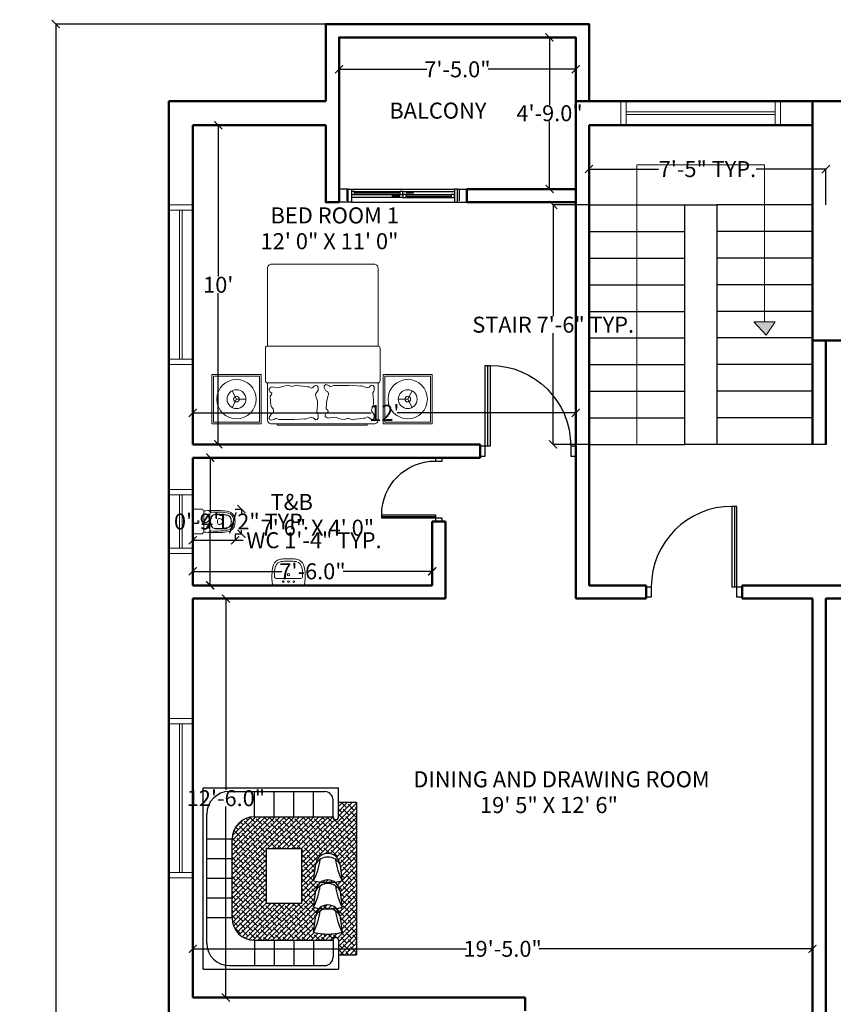
# Model space of a CAD drawing. Units: inches. Extents: x 147 to 1638, y 107 to 941.
# Tile 16 of 17: x 1062 to 1368, y 570 to 940. Entities that reach past the tile are written whole.
import ezdxf

# ---------------------------------------------------------------- set-up
doc = ezdxf.new("R2010")
doc.units = ezdxf.units.IN
doc.header["$MEASUREMENT"] = 0
for name, color, linetype, lineweight in [('A-ANNO-DIMS', 2, 'Continuous', 15), ('A-ANNO-SYMB', 7, 'Continuous', 18), ('A-AREA-IDEN', 7, 'Continuous', 18), ('A-Door', 150, 'Continuous', 25), ('A-FLOR-FIXT', 9, 'Continuous', 18), ('A-FLOR-STRS', 7, 'Continuous', 25), ('furniture', 50, 'Continuous', 18), ('HAT', 9, 'Continuous', 0), ('walls', 7, 'Continuous', 50), ('windows', 3, 'Continuous', 20)]:
    doc.layers.add(name, color=color, linetype=linetype, lineweight=lineweight)
for name, color, linetype in [('A-Glaz', 92, 'Continuous'), ('FUR', 42, 'Continuous'), ('NT', 1, 'Continuous'), ('Win', 152, 'Continuous')]:
    doc.layers.add(name, color=color, linetype=linetype)
doc.styles.get("Standard").update_dxf_attribs({"font": 'arial.ttf'})
doc.dimstyles.get("Standard").update_dxf_attribs({"dimtxt": 6, "dimasz": 3, "dimexe": 0.18, "dimexo": 0.0625, "dimgap": 0.09, "dimtad": 0, "dimtih": 1, "dimtoh": 1, "dimdec": 1, "dimzin": 0, "dimdsep": 46, "dimlunit": 3, "dimtxsty": 'Standard', "dimblk": 'ARCHTICK', "dimcen": 0.09, "dimadec": 0, "dimazin": 0, "dimtfac": 1, "dimtdec": 1, "dimtofl": 0, "dimtmove": 0, "dimatfit": 3, "dimfxl": 1, "dimtolj": 1, "dimtzin": 0, "dimarcsym": 0})

# ---------------------------------------------------------------- blocks, each defined once
blk = doc.blocks.new('A$C087A3AA9')
at = {"layer": 'A-Door'}
for points in [[(852.6, 94.7), (852.6, 852.6), (805.3, 852.6), (805.3, 94.7)], [(47.4, 94.7), (47.4, 0), (0, 0), (0, 94.7)], [(900, 94.7), (900, 0), (852.6, 0), (852.6, 94.7)]]:
    blk.add_lwpolyline(points, close=True, dxfattribs=at)
at = {"layer": 'A-Glaz'}
blk.add_line((828.9, 852.6), (828.9, 94.7), dxfattribs=at)
at = {"layer": 'NT'}
blk.add_arc((805.3, 94.7), 757.9, 90, 180, dxfattribs=at)
blk = doc.blocks.new('_ArchTick')
at = {"color": 0, "linetype": 'ByBlock', "const_width": 0.15}
blk.add_lwpolyline([(-0.5, -0.5), (0.5, 0.5)], dxfattribs=at)
blk = doc.blocks.new('*D49')
at = {"layer": 'A-ANNO-DIMS', "color": 0, "lineweight": -2, "transparency": 16777216}
for p, q in [((1132.08, 900.72), (1136.52, 900.72)), ((1136.34, 900.72), (1136.34, 843.87)), ((1136.34, 780.72), (1136.34, 837.56)), ((1132.08, 780.72), (1136.52, 780.72))]:
    blk.add_line(p, q, dxfattribs=at)
at = {"layer": 'Defpoints', "color": 0, "lineweight": -2, "transparency": 16777216}
for p in [(1132.02, 900.72), (1132.02, 780.72), (1136.34, 780.72)]:
    blk.add_point(p, dxfattribs=at)
at = {"layer": 'A-ANNO-DIMS', "color": 0, "lineweight": -2, "transparency": 16777216, "xscale": 3, "yscale": 3, "zscale": 3}
for p, rotation in [((1136.34, 900.72), 90), ((1136.34, 780.72), 270)]:
    blk.add_blockref('_ArchTick', p, dxfattribs=dict(at, rotation=rotation))
at = {"layer": 'A-ANNO-DIMS', "color": 0, "transparency": 16777216, "insert": (1136.34, 840.72), "char_height": 6, "attachment_point": 5}
blk.add_mtext("\\A1;10'", dxfattribs=at)
blk = doc.blocks.new('*D50')
at = {"layer": 'A-ANNO-DIMS', "color": 0, "lineweight": -2, "transparency": 16777216}
for p, q in [((1126.77, 788.89), (1126.77, 792.75)), ((1126.77, 792.57), (1193.87, 792.57)), ((1270.77, 792.57), (1203.67, 792.57)), ((1270.77, 788.89), (1270.77, 792.75))]:
    blk.add_line(p, q, dxfattribs=at)
at = {"layer": 'Defpoints', "color": 0, "lineweight": -2, "transparency": 16777216}
for p in [(1270.77, 792.57), (1126.77, 788.82), (1270.77, 788.82)]:
    blk.add_point(p, dxfattribs=at)
at = {"layer": 'A-ANNO-DIMS', "color": 0, "lineweight": -2, "transparency": 16777216, "xscale": 3, "yscale": 3, "zscale": 3, "rotation": 180}
blk.add_blockref('_ArchTick', (1126.77, 792.57), dxfattribs=at)
at = {"layer": 'A-ANNO-DIMS', "color": 0, "lineweight": -2, "transparency": 16777216, "xscale": 3, "yscale": 3, "zscale": 3}
blk.add_blockref('_ArchTick', (1270.77, 792.57), dxfattribs=at)
at = {"layer": 'A-ANNO-DIMS', "color": 0, "transparency": 16777216, "insert": (1198.77, 792.57), "char_height": 6, "attachment_point": 5}
blk.add_mtext("\\A1;12'", dxfattribs=at)
blk = doc.blocks.new('*D51')
at = {"layer": 'A-ANNO-DIMS', "color": 0, "lineweight": -2, "transparency": 16777216}
for p, q in [((1266.32, 933.72), (1260.72, 933.72)), ((1260.9, 933.72), (1260.9, 908.37)), ((1260.9, 876.72), (1260.9, 902.06)), ((1266.32, 876.72), (1260.72, 876.72))]:
    blk.add_line(p, q, dxfattribs=at)
at = {"layer": 'Defpoints', "color": 0, "lineweight": -2, "transparency": 16777216}
for p in [(1266.38, 933.72), (1260.9, 876.72), (1266.38, 876.72)]:
    blk.add_point(p, dxfattribs=at)
at = {"layer": 'A-ANNO-DIMS', "color": 0, "lineweight": -2, "transparency": 16777216, "xscale": 3, "yscale": 3, "zscale": 3}
for p, rotation in [((1260.9, 933.72), 90), ((1260.9, 876.72), 270)]:
    blk.add_blockref('_ArchTick', p, dxfattribs=dict(at, rotation=rotation))
at = {"layer": 'A-ANNO-DIMS', "color": 0, "transparency": 16777216, "insert": (1260.9, 905.22), "char_height": 6, "attachment_point": 5}
blk.add_mtext('\\A1;4\'-9.0"', dxfattribs=at)
blk = doc.blocks.new('*D52')
at = {"layer": 'A-ANNO-DIMS', "color": 0, "lineweight": -2, "transparency": 16777216}
for p, q in [((1181.77, 928.29), (1181.77, 921.54)), ((1270.77, 928.29), (1270.77, 921.54)), ((1181.77, 921.72), (1214.73, 921.72)), ((1270.77, 921.72), (1237.8, 921.72))]:
    blk.add_line(p, q, dxfattribs=at)
at = {"layer": 'Defpoints', "color": 0, "lineweight": -2, "transparency": 16777216}
for p in [(1181.77, 928.35), (1270.77, 928.35), (1270.77, 921.72)]:
    blk.add_point(p, dxfattribs=at)
at = {"layer": 'A-ANNO-DIMS', "color": 0, "lineweight": -2, "transparency": 16777216, "xscale": 3, "yscale": 3, "zscale": 3, "rotation": 180}
blk.add_blockref('_ArchTick', (1181.77, 921.72), dxfattribs=at)
at = {"layer": 'A-ANNO-DIMS', "color": 0, "lineweight": -2, "transparency": 16777216, "xscale": 3, "yscale": 3, "zscale": 3}
blk.add_blockref('_ArchTick', (1270.77, 921.72), dxfattribs=at)
at = {"layer": 'A-ANNO-DIMS', "color": 0, "transparency": 16777216, "insert": (1226.27, 921.72), "char_height": 6, "attachment_point": 5}
blk.add_mtext('\\A1;7\'-5.0"', dxfattribs=at)
blk = doc.blocks.new('*D55')
at = {"layer": 'A-ANNO-DIMS', "color": 0, "lineweight": -2, "transparency": 16777216}
for p, q in [((1126.77, 733.06), (1126.77, 733.17)), ((1126.77, 732.99), (1160.23, 732.99)), ((1216.77, 732.99), (1183.3, 732.99)), ((1216.77, 733.06), (1216.77, 733.17))]:
    blk.add_line(p, q, dxfattribs=at)
at = {"layer": 'Defpoints', "color": 0, "lineweight": -2, "transparency": 16777216}
for p in [(1126.77, 732.99), (1216.77, 732.99), (1216.77, 732.99)]:
    blk.add_point(p, dxfattribs=at)
at = {"layer": 'A-ANNO-DIMS', "color": 0, "lineweight": -2, "transparency": 16777216, "xscale": 3, "yscale": 3, "zscale": 3, "rotation": 180}
blk.add_blockref('_ArchTick', (1126.77, 732.99), dxfattribs=at)
at = {"layer": 'A-ANNO-DIMS', "color": 0, "lineweight": -2, "transparency": 16777216, "xscale": 3, "yscale": 3, "zscale": 3}
blk.add_blockref('_ArchTick', (1216.77, 732.99), dxfattribs=at)
at = {"layer": 'A-ANNO-DIMS', "color": 0, "transparency": 16777216, "insert": (1171.77, 732.99), "char_height": 6, "attachment_point": 5}
blk.add_mtext('\\A1;7\'-6.0"', dxfattribs=at)
blk = doc.blocks.new('*D56')
at = {"layer": 'A-ANNO-DIMS', "color": 0, "lineweight": -2, "transparency": 16777216}
for p, q in [((1133.31, 775.72), (1133.31, 754.81)), ((1133.37, 775.72), (1133.49, 775.72)), ((1133.31, 727.72), (1133.31, 748.63)), ((1133.37, 727.72), (1133.49, 727.72))]:
    blk.add_line(p, q, dxfattribs=at)
at = {"layer": 'Defpoints', "color": 0, "lineweight": -2, "transparency": 16777216}
for p in [(1133.31, 775.72), (1133.31, 727.72), (1133.31, 727.72)]:
    blk.add_point(p, dxfattribs=at)
at = {"layer": 'A-ANNO-DIMS', "color": 0, "lineweight": -2, "transparency": 16777216, "xscale": 3, "yscale": 3, "zscale": 3}
for p, rotation in [((1133.31, 775.72), 90), ((1133.31, 727.72), 270)]:
    blk.add_blockref('_ArchTick', p, dxfattribs=dict(at, rotation=rotation))
at = {"layer": 'A-ANNO-DIMS', "color": 0, "transparency": 16777216, "insert": (1133.31, 751.72), "char_height": 6, "attachment_point": 5}
blk.add_mtext("\\A1;4'", dxfattribs=at)
blk = doc.blocks.new('*D57')
at = {"layer": 'A-ANNO-DIMS', "color": 0, "lineweight": -2, "transparency": 16777216}
for p, q in [((1140.05, 722.72), (1139.05, 722.72)), ((1139.23, 722.72), (1139.23, 650.87)), ((1139.23, 572.72), (1139.23, 644.56)), ((1140.05, 572.72), (1139.05, 572.72))]:
    blk.add_line(p, q, dxfattribs=at)
at = {"layer": 'Defpoints', "color": 0, "lineweight": -2, "transparency": 16777216}
for p in [(1140.11, 722.72), (1139.23, 572.72), (1140.11, 572.72)]:
    blk.add_point(p, dxfattribs=at)
at = {"layer": 'A-ANNO-DIMS', "color": 0, "lineweight": -2, "transparency": 16777216, "xscale": 3, "yscale": 3, "zscale": 3}
for p, rotation in [((1139.23, 722.72), 90), ((1139.23, 572.72), 270)]:
    blk.add_blockref('_ArchTick', p, dxfattribs=dict(at, rotation=rotation))
at = {"layer": 'A-ANNO-DIMS', "color": 0, "transparency": 16777216, "insert": (1139.23, 647.72), "char_height": 6, "attachment_point": 5}
blk.add_mtext('\\A1;12\'-6.0"', dxfattribs=at)
blk = doc.blocks.new('*D58')
at = {"layer": 'A-ANNO-DIMS', "color": 0, "lineweight": -2, "transparency": 16777216}
for p, q in [((1126.77, 585.3), (1126.77, 591.26)), ((1126.77, 591.08), (1229.66, 591.08)), ((1359.77, 591.08), (1256.88, 591.08)), ((1359.77, 585.3), (1359.77, 591.26))]:
    blk.add_line(p, q, dxfattribs=at)
at = {"layer": 'Defpoints', "color": 0, "lineweight": -2, "transparency": 16777216}
for p in [(1359.77, 591.08), (1126.77, 585.23), (1359.77, 585.23)]:
    blk.add_point(p, dxfattribs=at)
at = {"layer": 'A-ANNO-DIMS', "color": 0, "lineweight": -2, "transparency": 16777216, "xscale": 3, "yscale": 3, "zscale": 3, "rotation": 180}
blk.add_blockref('_ArchTick', (1126.77, 591.08), dxfattribs=at)
at = {"layer": 'A-ANNO-DIMS', "color": 0, "lineweight": -2, "transparency": 16777216, "xscale": 3, "yscale": 3, "zscale": 3}
blk.add_blockref('_ArchTick', (1359.77, 591.08), dxfattribs=at)
at = {"layer": 'A-ANNO-DIMS', "color": 0, "transparency": 16777216, "insert": (1243.27, 591.08), "char_height": 6, "attachment_point": 5}
blk.add_mtext('\\A1;19\'-5.0"', dxfattribs=at)
blk = doc.blocks.new('MAT-P14')
for p, q in [((-1.337, 1.348), (-1.337, 1.948)), ((-1.337, 1.948), (-0.737, 1.948)), ((-1.317, 1.928), (-0.757, 1.928)), ((-1.317, 1.368), (-1.317, 1.928)), ((-0.757, 1.368), (-0.757, 1.928)), ((-0.737, 1.348), (-0.737, 1.948)), ((0.625, 1.95), (-0.625, 1.95)), ((0.753, 1.348), (0.753, 1.948)), ((1.353, 1.948), (0.753, 1.948)), ((1.333, 1.928), (0.773, 1.928)), ((0.773, 1.368), (0.773, 1.928)), ((1.333, 1.368), (1.333, 1.928)), ((1.353, 1.348), (1.353, 1.948)), ((-1.037, 1.648), (-1.091, 1.749)), ((1.053, 1.648), (1.108, 1.749)), ((-1.037, 1.648), (-1.091, 1.547)), ((-1.037, 1.648), (-0.922, 1.648)), ((1.053, 1.648), (0.938, 1.648)), ((1.053, 1.648), (1.108, 1.547)), ((-1.337, 1.348), (-0.737, 1.348)), ((-1.317, 1.368), (-0.757, 1.368)), ((1.353, 1.348), (0.753, 1.348)), ((1.333, 1.368), (0.773, 1.368))]:
    blk.add_line(p, q)
for points in [[(-0.675, 1.45), (-0.675, 1.9, -0.414214), (-0.625, 1.95), (0.625, 1.95, -0.414214), (0.675, 1.9), (0.675, 1.45)], [(-0.675, 1, -0.414214), (-0.7, 1.025), (-0.7, 1.425, -0.414214), (-0.675, 1.45), (0.675, 1.45, -0.414214), (0.7, 1.425), (0.7, 1.025, -0.414214), (0.675, 1)], [(-0.625, 0, -0.414214), (-0.675, 0.05), (-0.675, 1), (0.675, 1), (0.675, 0.05, -0.414214), (0.625, 0)]]:
    blk.add_lwpolyline(points, format="xyb", close=True)
blk.add_lwpolyline([(-0.542, 1.95), (-0.542, 1.967), (0.558, 1.967), (0.558, 1.95)], close=True)
for points in [[(-0.614, 1.818), (-0.626, 1.838), (-0.626, 1.877), (-0.614, 1.891), (-0.596, 1.896), (-0.579, 1.886), (-0.563, 1.872), (-0.545, 1.863), (-0.516, 1.879), (-0.497, 1.882), (-0.465, 1.884), (-0.439, 1.887), (-0.395, 1.892), (-0.363, 1.9), (-0.309, 1.882), (-0.262, 1.897), (-0.23, 1.892), (-0.192, 1.884), (-0.166, 1.873), (-0.128, 1.868), (-0.082, 1.875), (-0.076, 1.88), (-0.052, 1.875), (-0.028, 1.861), (-0.028, 1.841), (-0.04, 1.817), (-0.064, 1.802), (-0.06, 1.781), (-0.043, 1.768), (-0.046, 1.697), (-0.05, 1.662), (-0.056, 1.64), (-0.062, 1.612), (-0.068, 1.596), (-0.068, 1.579), (-0.063, 1.56), (-0.039, 1.545), (-0.015, 1.505), (-0.015, 1.486), (-0.038, 1.471), (-0.075, 1.482), (-0.081, 1.487), (-0.087, 1.497), (-0.134, 1.481), (-0.304, 1.482), (-0.318, 1.482), (-0.335, 1.479), (-0.464, 1.488), (-0.467, 1.486), (-0.473, 1.486), (-0.517, 1.503), (-0.53, 1.505), (-0.548, 1.51), (-0.566, 1.501), (-0.581, 1.487), (-0.599, 1.477), (-0.617, 1.482), (-0.629, 1.497), (-0.629, 1.536), (-0.623, 1.55), (-0.611, 1.57), (-0.614, 1.614), (-0.615, 1.627), (-0.618, 1.644), (-0.619, 1.66), (-0.62, 1.675), (-0.62, 1.695), (-0.618, 1.707), (-0.614, 1.723), (-0.608, 1.739), (-0.604, 1.75), (-0.598, 1.771), (-0.596, 1.785), (-0.6, 1.798), (-0.614, 1.819)], [(0.069, 1.559), (0.057, 1.54), (0.057, 1.501), (0.069, 1.486), (0.087, 1.481), (0.105, 1.491), (0.121, 1.505), (0.139, 1.514), (0.168, 1.498), (0.187, 1.496), (0.219, 1.493), (0.244, 1.49), (0.289, 1.485), (0.321, 1.477), (0.374, 1.495), (0.422, 1.48), (0.454, 1.486), (0.492, 1.493), (0.517, 1.504), (0.555, 1.509), (0.602, 1.502), (0.608, 1.497), (0.632, 1.502), (0.656, 1.517), (0.656, 1.536), (0.644, 1.561), (0.62, 1.575), (0.624, 1.596), (0.641, 1.609), (0.637, 1.68), (0.633, 1.715), (0.628, 1.738), (0.606, 1.765), (0.6, 1.781), (0.6, 1.798), (0.605, 1.817), (0.629, 1.832), (0.654, 1.872), (0.654, 1.892), (0.63, 1.906), (0.593, 1.895), (0.587, 1.891), (0.581, 1.881), (0.534, 1.896), (0.379, 1.896), (0.366, 1.896), (0.348, 1.898), (0.22, 1.89), (0.216, 1.891), (0.21, 1.891), (0.167, 1.875), (0.154, 1.872), (0.136, 1.867), (0.118, 1.876), (0.102, 1.89), (0.085, 1.9), (0.067, 1.895), (0.055, 1.881), (0.055, 1.842), (0.061, 1.827), (0.073, 1.807), (0.07, 1.764), (0.069, 1.75), (0.066, 1.733), (0.065, 1.718), (0.063, 1.703), (0.063, 1.682), (0.066, 1.67), (0.07, 1.655), (0.075, 1.638), (0.079, 1.627), (0.086, 1.607), (0.087, 1.592), (0.083, 1.579), (0.07, 1.559)]]:
    blk.add_lwpolyline(points)
for centre, radius in [((-1.037, 1.648), 0.24), ((1.053, 1.648), 0.24), ((-1.037, 1.648), 0.115), ((-1.037, 1.648), 0.035), ((1.053, 1.648), 0.115), ((1.053, 1.648), 0.035)]:
    blk.add_circle(centre, radius)
blk = doc.blocks.new('2SAINDA')
at = {"color": 0, "linetype": 'ByBlock'}
for p, q in [((0, 0.188), (0, -0.188)), ((0.018, 0.2), (0.141, 0.2)), ((0.157, 0.192), (0.162, 0.188)), ((0.18, -0.164), (0.18, 0.164)), ((0.279, 0.159), (0.261, 0.176)), ((0.437, 0.047), (0.424, 0.047)), ((0.279, -0.159), (0.261, -0.176)), ((0.437, -0.047), (0.424, -0.047)), ((0.018, -0.2), (0.141, -0.2)), ((0.157, -0.192), (0.162, -0.188))]:
    blk.add_line(p, q, dxfattribs=at)
for centre, radius in [((0.09, 0), 0.0135), ((0.09, 0), 0.0135), ((0.236, 0.08), 0.0075), ((0.236, -0.08), 0.0075)]:
    blk.add_circle(centre, radius, dxfattribs=at)
for centre, radius, start, end in [((0.018, 0.18), 0.02, 90, 155.6901), ((0.141, 0.181), 0.019, 34.9372, 90), ((0.155, 0.164), 0.025, 23.3776, 73.7848), ((0.383, -5.322), 5.5, 89.2905, 92.1362), ((0.155, 0.164), 0.025, 360, 23.3776), ((0.444, -0.373), 0.55, 75.4605, 89.2905), ((0.549, 0.03), 0.134, 8.8162, 75.4605), ((0.293, 0.173), 0.02, 225, 270.9364), ((0.485, 0), 0.2, 160.016, 199.984), ((0.485, 0), 0.196, 160.016, 199.984), ((0.383, -5.322), 5.476, 89.2905, 90.9364), ((0.368, 0.043), 0.075, 90.1648, 160.016), ((0.368, 0.043), 0.071, 90.1648, 160.016), ((0.383, -5.322), 5.44, 89.2905, 90.1648), ((0.383, -5.322), 5.436, 89.2905, 90.1648), ((0.582, 0), 0.18, 170.2849, 189.7151), ((0.424, 0.027), 0.02, 90, 170.2849), ((0.437, 0), 0.047, 0, 90), ((0.437, 0), 0.047, 270, 0), ((0.444, -0.373), 0.49, 75.4605, 89.2905), ((0.444, -0.373), 0.486, 75.4605, 89.2905), ((0.444, -0.373), 0.526, 75.4605, 89.2905), ((0.549, 0.03), 0.07, 8.8162, 75.4605), ((0.549, 0.03), 0.074, 8.8162, 75.4605), ((0.549, 0.03), 0.11, 8.8162, 75.4605), ((0.355, 0), 0.266, 351.1838, 8.8162), ((0.355, 0), 0.27, 351.1838, 8.8162), ((0.355, 0), 0.306, 351.1838, 8.8162), ((0.355, 0), 0.33, 351.1838, 8.8162), ((0.293, -0.173), 0.02, 89.0636, 135), ((0.383, 5.322), 5.476, 269.0636, 270.7095), ((0.368, -0.043), 0.075, 199.984, 269.8352), ((0.368, -0.043), 0.071, 199.984, 269.8352), ((0.383, 5.322), 5.436, 269.8352, 270.7095), ((0.383, 5.322), 5.44, 269.8352, 270.7095), ((0.424, -0.027), 0.02, 189.7151, 270), ((0.444, 0.373), 0.486, 270.7095, 284.5395), ((0.444, 0.373), 0.49, 270.7095, 284.5395), ((0.444, 0.373), 0.526, 270.7095, 284.5395), ((0.549, -0.03), 0.07, 284.5395, 351.1838), ((0.549, -0.03), 0.074, 284.5395, 351.1838), ((0.549, -0.03), 0.11, 284.5395, 351.1838), ((0.549, -0.03), 0.134, 284.5395, 351.1838), ((0.018, -0.18), 0.02, 204.3099, 270), ((0.141, -0.181), 0.019, 270, 325.0628), ((0.155, -0.164), 0.025, 286.2152, 336.6224), ((0.155, -0.164), 0.025, 336.6224, 0), ((0.383, 5.322), 5.5, 267.8638, 270.7095), ((0.444, 0.373), 0.55, 270.7095, 284.5395)]:
    blk.add_arc(centre, radius, start, end, dxfattribs=at)
blk = doc.blocks.new('2SALADA2')
at = {"color": 0}
for p, q in [((-0.296, 0), (0.296, 0)), ((0.207, -0.13), (-0.207, -0.13))]:
    blk.add_line(p, q, dxfattribs=at)
for centre, radius in [((-0.1, -0.07), 0.015), ((0, -0.205), 0.023), ((0, -0.07), 0.0175), ((0.1, -0.07), 0.015)]:
    blk.add_circle(centre, radius, dxfattribs=at)
for centre, radius, start, end in [((-0.296, -0.01), 0.01, 90, 173.6262), ((0.296, -0.01), 0.01, 6.3738, 90), ((1.185, -0.175), 1.5, 173.6262, 182.693), ((1.186, -0.221), 1.454, 178.0234, 180.898), ((-0.227, -0.171), 0.04, 95.5937, 179.6995), ((-0.207, -0.38), 0.25, 90, 95.5937), ((0.207, -0.38), 0.25, 84.4063, 90), ((0.227, -0.171), 0.04, 0.3005, 84.4063), ((-1.186, -0.221), 1.454, 359.102, 1.9766), ((-1.185, -0.175), 1.5, 357.307, 6.3738), ((0.186, -0.222), 0.5, 182.693, 199.3406), ((0.186, -0.222), 0.454, 182.693, 199.3406), ((-0.135, -0.335), 0.114, 199.3406, 257.4429), ((0.135, -0.335), 0.114, 282.5571, 340.6594), ((-0.186, -0.222), 0.454, 340.6594, 357.307), ((-0.186, -0.222), 0.5, 340.6594, 357.307), ((-0.135, -0.335), 0.16, 199.3406, 257.4429), ((-0.061, -0.003), 0.5, 257.4429, 266.4982), ((-0.061, -0.003), 0.454, 257.4429, 266.4982), ((0, 0.995), 1.5, 266.4982, 273.5018), ((0, 0.995), 1.454, 266.4982, 273.5018), ((0.061, -0.003), 0.454, 273.5018, 282.5571), ((0.061, -0.003), 0.5, 273.5018, 282.5571), ((0.135, -0.335), 0.16, 282.5571, 340.6594)]:
    blk.add_arc(centre, radius, start, end, dxfattribs=at)
blk = doc.blocks.new('CHAIR1')
for p, q in [((-393, -750), (-329, -287)), ((329, -286), (394, -750))]:
    blk.add_line(p, q)
for centre, radius, start, end in [((0, -332), 332, 7.9072, 172.1612), ((-1856, 27), 1657, 332.0394, 353.4161), ((0, -483), 383, 30.9021, 149.1663), ((1857, 27), 1657, 186.5839, 207.9606), ((0, 770), 1570, 255.502, 284.498)]:
    blk.add_arc(centre, radius, start, end)
blk = doc.blocks.new('A$C1CFC4E3A')
at = {"layer": 'HAT'}
h = blk.add_hatch(dxfattribs=at)
h.set_pattern_fill('ANSI38,_O', color=256, scale=0.664121)
h.set_pattern_definition([(45, (6.13299, -18.48134), (-0.05870057, 0.05870057), []), (135, (6.13299, -18.48134), (-0.1761017, 0.05870057), [0.2075378, -0.1245227])])
h.paths.add_polyline_path([(0, 3.705), (-0.438, 3.705), (-0.438, 3.353, -1), (-0.573, 3.353), (-2.482, 3.353, 0.414214), (-3.028, 2.807), (-3.028, 0.898, 0.414214), (-2.482, 0.352), (-0.573, 0.352, -1), (-0.438, 0.352), (-0.438, 0), (0, 0)])
h.paths.add_polyline_path([(-1.342, 1.248), (-2.191, 1.248), (-2.191, 2.58), (-1.342, 2.58)], flags=16)
h.paths.add_polyline_path([(-0.409, 1.566), (-0.352, 1.156, -0.127199), (-1.048, 1.156), (-0.992, 1.566, -0.871235)], flags=16)
h.paths.add_polyline_path([(-0.409, 0.959), (-0.352, 0.548, -0.127199), (-1.048, 0.548), (-0.992, 0.958, -0.871235)], flags=16)
h.paths.add_polyline_path([(-0.992, 2.209, -0.871235), (-0.409, 2.21), (-0.352, 1.799, -0.127199), (-1.048, 1.799)], flags=16)
at = {"layer": 'FUR'}
for p, q in [((-3.732, 4.057), (-0.438, 4.057)), ((-3.732, -0.352), (-3.732, 4.057)), ((-3.096, 3.967), (-0.777, 3.967)), ((-2.482, 3.353), (-2.482, 3.967)), ((-2.005, 3.353), (-2.005, 3.967)), ((-1.528, 3.353), (-1.528, 3.967)), ((-1.05, 3.353), (-1.05, 3.967)), ((-0.438, 3.353), (-0.438, 4.057)), ((-0.573, 3.353), (-0.573, 3.762)), ((-3.642, 0.284), (-3.642, 3.421)), ((-2.482, 3.353), (-0.573, 3.353)), ((-3.028, 2.807), (-3.642, 2.807)), ((-3.028, 2.33), (-3.642, 2.33)), ((-3.028, 1.852), (-3.642, 1.852)), ((-3.028, 1.375), (-3.642, 1.375)), ((-3.028, 0.898), (-3.642, 0.898)), ((-2.482, 0.352), (-0.573, 0.352)), ((-2.482, 0.352), (-2.482, -0.262)), ((-2.005, 0.352), (-2.005, -0.262)), ((-1.528, 0.352), (-1.528, -0.262)), ((-1.05, 0.352), (-1.05, -0.262)), ((-0.573, 0.352), (-0.573, -0.057)), ((-0.438, 0.352), (-0.438, -0.352)), ((-3.732, -0.352), (-0.438, -0.352)), ((-3.096, -0.262), (-0.777, -0.262))]:
    blk.add_line(p, q, dxfattribs=at)
for centre, radius, start, end in [((-3.096, 3.421), 0.546, 90, 180), ((-0.777, 3.762), 0.205, 0, 90), ((-2.482, 2.807), 0.546, 90, 180), ((-0.505, 3.353), 0.0675, 180, 0), ((-2.482, 0.898), 0.546, 180, 270), ((-3.096, 0.284), 0.546, 180, 270), ((-0.505, 0.352), 0.0675, 0, 180), ((-0.777, -0.057), 0.205, 270, 0)]:
    blk.add_arc(centre, radius, start, end, dxfattribs=at)
at = {"layer": 'Win'}
for p, q in [((-0.438, 3.705), (0, 3.705)), ((0, 3.705), (0, 0)), ((-3.028, 0.898), (-3.028, 2.807)), ((-0.438, 0), (0, 0))]:
    blk.add_line(p, q, dxfattribs=at)
blk.add_lwpolyline([(-2.191, 2.58), (-1.342, 2.58), (-1.342, 1.248), (-2.191, 1.248)], close=True, dxfattribs=at)
at = {"layer": 'FUR', "xscale": 0.0008854948152227, "yscale": 0.0008854948152227, "zscale": 0.0008854948152227}
for p in [(-0.7, 2.463), (-0.7, 1.82), (-0.7, 1.212)]:
    blk.add_blockref('CHAIR1', p, dxfattribs=at)
blk = doc.blocks.new('WIN-60IN')
for p, q in [((60, 9), (0, 9)), ((0, 9), (0, 0)), ((2, 9), (2, 0)), ((58, 0), (58, 9)), ((60, 0), (60, 9)), ((2, 5), (58, 5)), ((2, 4), (58, 4)), ((0, 0), (60, 0))]:
    blk.add_line(p, q)
blk = doc.blocks.new('WIN-24IN')
for p, q in [((9, 24), (0, 24)), ((0, 24), (0, 0)), ((9, 0), (9, 24)), ((9, 22), (0, 22)), ((4, 2), (4, 22)), ((5, 2), (5, 22)), ((0, 2), (9, 2)), ((0, 0), (9, 0))]:
    blk.add_line(p, q)
blk = doc.blocks.new('DOOR-SLIDING-48IN')
for p, q in [((3.46, 5), (0, 5)), ((2.87, 5), (2.87, 0.59)), ((3.46, 0), (3.46, 5)), ((3.46, 5), (4.63, 5)), ((4.63, 5), (43.37, 5)), ((4.63, 5), (4.63, 0)), ((5.81, 4.11), (22.83, 4.11)), ((24, 4.11), (43.37, 4.11)), ((44.54, 5), (43.37, 5)), ((43.37, 5), (43.37, 0)), ((44.54, 5), (48, 5)), ((44.54, 0), (44.54, 5)), ((45.13, 5), (45.13, 0.59)), ((3.46, 0), (0, 0)), ((4.63, 0), (3.46, 0)), ((24, 1.76), (4.63, 1.76)), ((4.63, 0), (43.37, 0)), ((5.81, 3.52), (22.83, 3.52)), ((5.81, 2.93), (22.83, 2.93)), ((22.83, 2.35), (20.3, 2.35)), ((25.17, 3.52), (27.7, 3.52)), ((25.17, 2.93), (42.19, 2.93)), ((25.17, 2.35), (42.19, 2.35)), ((25.17, 1.76), (42.19, 1.76)), ((43.37, 0), (44.54, 0)), ((44.54, 0), (48, 0))]:
    blk.add_line(p, q)
for points in [[(4.63, 2.93), (5.81, 2.93), (5.81, 4.11), (4.63, 4.11)], [(22.83, 2.93), (24, 2.93), (24, 4.11), (22.83, 4.11)], [(20, 2.35), (20.3, 2.52), (20.3, 2.17)], [(24, 1.76), (25.17, 1.76), (25.17, 2.93), (24, 2.93)], [(28, 3.52), (27.7, 3.7), (27.7, 3.35)], [(42.19, 1.76), (43.37, 1.76), (43.37, 2.93), (42.19, 2.93)]]:
    blk.add_lwpolyline(points, close=True)
blk = doc.blocks.new('STAIR-RETURN-FLIGHTS')
for p, q in [((0, 90), (36, 90)), ((36, 0), (36, 90)), ((36, 90), (48, 90)), ((84, 90), (48, 90)), ((48, 90), (48, 0)), ((0, 80), (36, 80)), ((84, 80), (48, 80)), ((0, 70), (36, 70)), ((84, 70), (48, 70)), ((0, 60), (36, 60)), ((84, 60), (48, 60)), ((0, 50), (36, 50)), ((84, 50), (48, 50)), ((0, 40), (36, 40)), ((84, 40), (48, 40)), ((0, 30), (36, 30)), ((84, 30), (48, 30)), ((0, 20), (36, 20)), ((84, 20), (48, 20)), ((0, 10), (36, 10)), ((84, 10), (48, 10)), ((0, 0), (36, 0)), ((48, 0), (36, 0)), ((89, 0), (48, 0))]:
    blk.add_line(p, q)
blk = doc.blocks.new('STAIR-DIRECTION-RETURN')
h = blk.add_hatch(color=256)
h.dxf.hatch_style = 1
h.paths.add_polyline_path([(52, 46.08), (48, 46.08), (44, 46.08), (48.61, 41.07)])
for p, q in [((0, 0), (0, 105.11)), ((0, 105.11), (48, 105.11)), ((48, 105.11), (48, 46.08)), ((48, 46.08), (44, 46.08)), ((48.61, 41.07), (44, 46.08)), ((48, 46.08), (52, 46.08)), ((52, 46.08), (48.61, 41.07))]:
    blk.add_line(p, q)
blk = doc.blocks.new('*D118')
at = {"layer": 'A-ANNO-DIMS', "color": 0, "lineweight": -2, "transparency": 16777216}
for p, q in [((1126.77, 747.02), (1126.77, 744.51)), ((1126.77, 744.69), (1142.68, 744.69)), ((1142.68, 747.02), (1142.68, 744.51)), ((1142.68, 744.69), (1145.68, 744.69))]:
    blk.add_line(p, q, dxfattribs=at)
at = {"layer": 'Defpoints', "color": 0, "lineweight": -2, "transparency": 16777216}
for p in [(1126.77, 747.08), (1142.68, 747.08), (1142.68, 744.69)]:
    blk.add_point(p, dxfattribs=at)
at = {"layer": 'A-ANNO-DIMS', "color": 0, "lineweight": -2, "transparency": 16777216, "xscale": 3, "yscale": 3, "zscale": 3, "rotation": 180}
blk.add_blockref('_ArchTick', (1126.77, 744.69), dxfattribs=at)
at = {"layer": 'A-ANNO-DIMS', "color": 0, "lineweight": -2, "transparency": 16777216, "xscale": 3, "yscale": 3, "zscale": 3}
blk.add_blockref('_ArchTick', (1142.68, 744.69), dxfattribs=at)
at = {"layer": 'A-ANNO-DIMS', "color": 0, "transparency": 16777216, "insert": (1172.33, 744.69), "char_height": 6, "attachment_point": 5}
blk.add_mtext('\\A1;WC 1\'-4" TYP.', dxfattribs=at)
blk = doc.blocks.new('*D119')
at = {"layer": 'A-ANNO-DIMS', "color": 0, "lineweight": -2, "transparency": 16777216}
for p, q in [((1142.75, 756.36), (1145.25, 756.36)), ((1145.07, 756.36), (1145.07, 754.91)), ((1145.07, 747.08), (1145.07, 748.53)), ((1142.75, 747.08), (1145.25, 747.08))]:
    blk.add_line(p, q, dxfattribs=at)
at = {"layer": 'Defpoints', "color": 0, "lineweight": -2, "transparency": 16777216}
for p in [(1142.68, 756.36), (1145.07, 756.36), (1142.68, 747.08)]:
    blk.add_point(p, dxfattribs=at)
at = {"layer": 'A-ANNO-DIMS', "color": 0, "lineweight": -2, "transparency": 16777216, "xscale": 3, "yscale": 3, "zscale": 3}
for p, rotation in [((1145.07, 756.36), 90), ((1145.07, 747.08), 270)]:
    blk.add_blockref('_ArchTick', p, dxfattribs=dict(at, rotation=rotation))
at = {"layer": 'A-ANNO-DIMS', "color": 0, "transparency": 16777216, "insert": (1145.07, 751.72), "char_height": 6, "attachment_point": 5}
blk.add_mtext('\\A1;0\'-9 1/2" TYP.', dxfattribs=at)
blk = doc.blocks.new('*D132')
at = {"layer": 'A-ANNO-DIMS', "color": 0, "lineweight": -2, "transparency": 16777216}
for p, q in [((1275.71, 870.72), (1262.09, 870.72)), ((1262.27, 870.72), (1262.27, 828.91)), ((1262.27, 780.72), (1262.27, 822.53)), ((1275.71, 780.72), (1262.09, 780.72))]:
    blk.add_line(p, q, dxfattribs=at)
at = {"layer": 'Defpoints', "color": 0, "lineweight": -2, "transparency": 16777216}
for p in [(1262.27, 870.72), (1275.77, 870.72), (1275.77, 780.72)]:
    blk.add_point(p, dxfattribs=at)
at = {"layer": 'A-ANNO-DIMS', "color": 0, "lineweight": -2, "transparency": 16777216, "xscale": 3, "yscale": 3, "zscale": 3}
for p, rotation in [((1262.27, 870.72), 90), ((1262.27, 780.72), 270)]:
    blk.add_blockref('_ArchTick', p, dxfattribs=dict(at, rotation=rotation))
at = {"layer": 'A-ANNO-DIMS', "color": 0, "transparency": 16777216, "insert": (1262.27, 825.72), "char_height": 6, "attachment_point": 5}
blk.add_mtext('\\A1;STAIR 7\'-6" TYP.', dxfattribs=at)
blk = doc.blocks.new('*D133')
at = {"layer": 'A-ANNO-DIMS', "color": 0, "lineweight": -2, "transparency": 16777216}
for p, q in [((1275.77, 870.78), (1275.77, 884.4)), ((1275.77, 884.22), (1301.92, 884.22)), ((1364.77, 884.22), (1338.62, 884.22)), ((1364.77, 870.78), (1364.77, 884.4))]:
    blk.add_line(p, q, dxfattribs=at)
at = {"layer": 'Defpoints', "color": 0, "lineweight": -2, "transparency": 16777216}
for p in [(1364.77, 884.22), (1275.77, 870.72), (1364.77, 870.72)]:
    blk.add_point(p, dxfattribs=at)
at = {"layer": 'A-ANNO-DIMS', "color": 0, "lineweight": -2, "transparency": 16777216, "xscale": 3, "yscale": 3, "zscale": 3, "rotation": 180}
blk.add_blockref('_ArchTick', (1275.77, 884.22), dxfattribs=at)
at = {"layer": 'A-ANNO-DIMS', "color": 0, "lineweight": -2, "transparency": 16777216, "xscale": 3, "yscale": 3, "zscale": 3}
blk.add_blockref('_ArchTick', (1364.77, 884.22), dxfattribs=at)
at = {"layer": 'A-ANNO-DIMS', "color": 0, "transparency": 16777216, "insert": (1320.27, 884.22), "char_height": 6, "attachment_point": 5}
blk.add_mtext('\\A1;7\'-5" TYP.', dxfattribs=at)
blk = doc.blocks.new('*D135')
at = {"layer": 'A-ANNO-DIMS', "color": 0, "lineweight": -2, "transparency": 16777216}
for p, q in [((1176.71, 938.72), (1075.09, 938.72)), ((1075.27, 938.72), (1075.27, 552.37)), ((1075.27, 159.72), (1075.27, 546.06)), ((1117.71, 159.72), (1075.09, 159.72))]:
    blk.add_line(p, q, dxfattribs=at)
at = {"layer": 'Defpoints', "color": 0, "lineweight": -2, "transparency": 16777216}
for p in [(1075.27, 938.72), (1176.77, 938.72), (1117.77, 159.72)]:
    blk.add_point(p, dxfattribs=at)
at = {"layer": 'A-ANNO-DIMS', "color": 0, "lineweight": -2, "transparency": 16777216, "xscale": 3, "yscale": 3, "zscale": 3}
for p, rotation in [((1075.27, 938.72), 90), ((1075.27, 159.72), 270)]:
    blk.add_blockref('_ArchTick', p, dxfattribs=dict(at, rotation=rotation))
at = {"layer": 'A-ANNO-DIMS', "color": 0, "transparency": 16777216, "insert": (1075.27, 549.22), "char_height": 6, "attachment_point": 5}
blk.add_mtext('\\A1;64\'-11"', dxfattribs=at)

msp = doc.modelspace()

# ---------------------------------------------------------------- linework, layer by layer
at = {"layer": 'walls'}
for p, q in [((1117.77, 909.72), (1117.77, 201.72)), ((1117.77, 909.72), (1176.77, 909.72)), ((1270.77, 900.72), (1270.77, 909.72)), ((1270.77, 909.72), (1441.77, 909.72)), ((1359.77, 909.72), (1359.77, 780.72)), ((1126.77, 900.72), (1126.77, 780.72)), ((1126.77, 900.72), (1176.77, 900.72)), ((1270.77, 900.72), (1270.77, 780.72)), ((1275.77, 900.72), (1275.77, 727.72)), ((1275.77, 900.72), (1359.77, 900.72)), ((1181.77, 876.72), (1181.77, 871.72)), ((1229.77, 876.72), (1229.77, 871.72)), ((1359.77, 819.72), (1388.77, 819.72)), ((1364.77, 819.72), (1364.77, 780.72)), ((1126.77, 780.72), (1234.77, 780.72)), ((1234.77, 780.72), (1234.77, 775.72)), ((1270.77, 780.72), (1270.77, 775.72)), ((1126.77, 775.72), (1126.77, 727.72)), ((1126.77, 775.72), (1216.77, 775.72)), ((1216.77, 775.72), (1221.77, 775.72)), ((1221.77, 775.72), (1234.77, 775.72)), ((1270.77, 775.72), (1270.77, 722.72)), ((1216.77, 751.72), (1216.77, 727.72)), ((1216.77, 751.72), (1221.77, 751.72)), ((1221.77, 751.72), (1221.77, 722.72)), ((1126.77, 727.72), (1216.77, 727.72)), ((1275.77, 727.72), (1297.27, 727.72)), ((1297.27, 722.72), (1297.27, 727.72)), ((1333.27, 727.72), (1385.27, 727.72)), ((1333.27, 722.72), (1333.27, 727.72)), ((1126.77, 722.72), (1126.77, 572.72)), ((1126.77, 722.72), (1221.77, 722.72)), ((1270.77, 722.72), (1297.27, 722.72)), ((1333.27, 722.72), (1359.77, 722.72)), ((1359.77, 722.72), (1359.77, 400.72)), ((1364.77, 722.72), (1364.77, 400.72)), ((1364.77, 722.72), (1385.27, 722.72)), ((1126.77, 572.72), (1251.77, 572.72)), ((1251.77, 572.72), (1251.77, 567.72))]:
    msp.add_line(p, q, dxfattribs=at)
for points in [[(1275.77, 909.72), (1275.77, 938.72), (1176.77, 938.72), (1176.77, 909.72)], [(1270.77, 909.72), (1270.77, 933.72), (1181.77, 933.72), (1181.77, 900.72), (1181.77, 876.72)], [(1176.77, 900.72), (1176.77, 871.72), (1181.77, 871.72)], [(1229.77, 876.72), (1270.77, 876.72)], [(1229.77, 871.72), (1270.77, 871.72)]]:
    msp.add_lwpolyline(points, dxfattribs=at)

# ---------------------------------------------------------------- block references
at = {"layer": 'A-ANNO-SYMB'}
msp.add_blockref('STAIR-DIRECTION-RETURN', (1293.77, 780.72), dxfattribs=at)
at = {"layer": 'A-Door'}
msp.add_blockref('DOOR-SLIDING-48IN', (1181.77, 871.72), dxfattribs=at)
at = {"layer": 'A-Door', "yscale": 0.0400000000000001, "zscale": 0.0400000000000001}
for p, xscale in [((1270.77, 776.32), -0.0400000000000001), ((1297.27, 723.32), 0.0400000000000001)]:
    msp.add_blockref('A$C087A3AA9', p, dxfattribs=dict(at, xscale=xscale))
at = {"layer": 'A-Door', "xscale": -0.0266666667542921, "yscale": 0.0266666667542921, "zscale": 0.0266666667542921, "rotation": 90}
msp.add_blockref('A$C087A3AA9', (1220.53, 775.72), dxfattribs=at)
at = {"layer": 'A-FLOR-FIXT', "xscale": 23.19012112898009, "yscale": 23.19012112898009, "zscale": 23.19012112898009}
msp.add_blockref('2SAINDA', (1126.77, 751.72), dxfattribs=at)
at = {"layer": 'A-FLOR-FIXT', "xscale": 19.81841434140962, "yscale": 19.81841434140962, "zscale": 19.81841434140962, "rotation": 180}
msp.add_blockref('2SALADA2', (1162.77, 727.72), dxfattribs=at)
at = {"layer": 'A-FLOR-STRS'}
msp.add_blockref('STAIR-RETURN-FLIGHTS', (1275.77, 780.72), dxfattribs=at)
at = {"layer": 'furniture', "xscale": 30.80045642108221, "yscale": 30.80045642108221, "zscale": 30.80045642108221, "rotation": 180}
msp.add_blockref('MAT-P14', (1175.64, 848.49), dxfattribs=at)
at = {"layer": 'furniture', "xscale": 15.47145176415956, "yscale": 15.47145176415956, "zscale": 15.47145176415956}
msp.add_blockref('A$C1CFC4E3A', (1188.37, 588.83), dxfattribs=at)
at = {"layer": 'windows'}
for p, rotation in [((1347.77, 909.72), 180), ((1117.77, 870.72), 270.0000000000011), ((1117.77, 677.72), 270.0000000000011)]:
    msp.add_blockref('WIN-60IN', p, dxfattribs=dict(at, rotation=rotation))
msp.add_blockref('WIN-24IN', (1117.77, 739.72), dxfattribs=at)

# ---------------------------------------------------------------- texts
at = {"layer": 'A-AREA-IDEN'}
for s, height, p in [('BALCONY', 6.031, (1200.65, 903.18)), ('BED ROOM 1', 6.031, (1156, 863.78)), ('  12\' 0" X 11\' 0"', 6.0306, (1148.55, 854.09)), ('T&B', 6.031, (1156, 756.05)), ('  7\' 6" X 4\' 0"', 6.0306, (1148.55, 746.37)), ('DINING AND DRAWING ROOM', 6.0306, (1209.68, 651.8)), ('19\' 5" X 12\' 6"', 6.0306, (1234.75, 642.11))]:
    msp.add_text(s, height=height, dxfattribs=at).set_placement(p)

# ---------------------------------------------------------------- dimensions: what is measured, and where the dimension line sits
at = {"layer": 'A-ANNO-DIMS'}
for base, p1, p2, override, picture, middle in [((1075.27, 938.72), (1117.77, 159.72), (1176.77, 938.72), {"dimdec": 1, "dimlfac": 1, "dimrnd": 0, "dimzin": 1, "dimdsep": 46, "dimlunit": 4, "dimfrac": 2}, '*D135', (1075.27, 549.22)), ((1260.9, 876.72), (1266.38, 933.72), (1266.38, 876.72), {"dimclrd": 0, "dimclre": 0, "dimclrt": 0}, '*D51', (1260.9, 905.22)), ((1136.34, 780.72), (1132.02, 900.72), (1132.02, 780.72), {"dimclrd": 0, "dimclre": 0, "dimclrt": 0}, '*D49', (1136.34, 840.72)), ((1133.31, 727.72), (1133.31, 775.72), (1133.31, 727.72), {"dimclrd": 0, "dimclre": 0, "dimclrt": 0}, '*D56', (1133.31, 751.72)), ((1139.23, 572.72), (1140.11, 722.72), (1140.11, 572.72), {"dimclrd": 0, "dimclre": 0, "dimclrt": 0}, '*D57', (1139.23, 647.72))]:
    dim = msp.add_linear_dim(base=base, p1=p1, p2=p2, angle=90, dimstyle='Standard', override=override, dxfattribs=at)
    dim.commit()
    dim.dimension.update_dxf_attribs({"geometry": picture, "text_midpoint": middle})
for base, p1, p2, picture, middle in [((1270.77, 921.72), (1181.77, 928.35), (1270.77, 928.35), '*D52', (1226.27, 921.72)), ((1270.77, 792.57), (1126.77, 788.82), (1270.77, 788.82), '*D50', (1198.77, 792.57)), ((1216.77, 732.99), (1126.77, 732.99), (1216.77, 732.99), '*D55', (1171.77, 732.99)), ((1359.77, 591.08), (1126.77, 585.23), (1359.77, 585.23), '*D58', (1243.27, 591.08))]:
    dim = msp.add_linear_dim(base=base, p1=p1, p2=p2, dimstyle='Standard', override={"dimclrd": 0, "dimclre": 0, "dimclrt": 0}, dxfattribs=at)
    dim.commit()
    dim.dimension.update_dxf_attribs({"geometry": picture, "text_midpoint": middle})
for base, p1, p2, text, picture, middle in [((1364.77, 884.22), (1275.77, 870.72), (1364.77, 870.72), '<> TYP.', '*D133', (1320.27, 884.22)), ((1142.68, 744.69), (1126.77, 747.08), (1142.68, 747.08), 'WC <> TYP.', '*D118', (1172.33, 744.69))]:
    dim = msp.add_linear_dim(base=base, p1=p1, p2=p2, text=text, dimstyle='Standard', override={"dimdec": 1, "dimlfac": 1, "dimrnd": 0, "dimzin": 1, "dimdsep": 46, "dimlunit": 4, "dimfrac": 2}, dxfattribs=at)
    dim.commit()
    dim.dimension.update_dxf_attribs({"geometry": picture, "text_midpoint": middle})
for base, p1, p2, text, picture, middle in [((1262.27, 870.72), (1275.77, 780.72), (1275.77, 870.72), 'STAIR <> TYP.', '*D132', (1262.27, 825.72)), ((1145.07, 756.36), (1142.68, 747.08), (1142.68, 756.36), '<> TYP.', '*D119', (1145.07, 751.72))]:
    dim = msp.add_linear_dim(base=base, p1=p1, p2=p2, angle=90, text=text, dimstyle='Standard', override={"dimdec": 1, "dimlfac": 1, "dimrnd": 0, "dimzin": 1, "dimdsep": 46, "dimlunit": 4, "dimfrac": 2}, dxfattribs=at)
    dim.commit()
    dim.dimension.update_dxf_attribs({"geometry": picture, "text_midpoint": middle})

doc.saveas('drawing.dxf')
